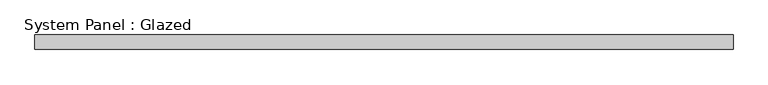
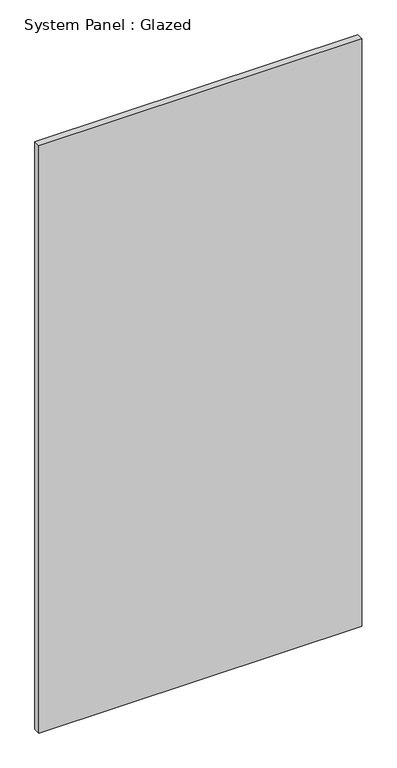
"""IFC4 building model written with IfcOpenShell, lengths in millimetres: plate geometry, System Panel : Glazed."""

from ifc_helpers import new_model, si_unit, origin, origin_with_axes, place, context, project, spatial, polyline, outline, extrude, source, transform, mapped, element, save


def system_panel_glazed_ecda40cd(model_context):
    return source(origin(), model_context, "Body", "SweptSolid", [
        extrude(outline(polyline([(609.5999999, -44.45), (-609.5999999, -44.45), (-609.5999999, -19.05), (609.5999999, -19.05), (609.5999999, -44.45)])), origin_with_axes(), (0.0, 0.0, 1.0), 2343.15),
    ])


if __name__ == "__main__":
    model = new_model("IFC4")
    model_context = context("Model", 3, world=origin())
    ifc_project = project(units=[si_unit("LENGTHUNIT", "METRE", prefix="MILLI")], contexts=[model_context])
    site = spatial("IfcSite", under=ifc_project)
    building = spatial("IfcBuilding", under=site)
    placement = place(None, origin())
    system_panel_glazed_shape = system_panel_glazed_ecda40cd(model_context)
    element("IfcPlate", 1, ObjectType="System Panel : Glazed", at=placement, inside=building, context=model_context, shape_type="MappedRepresentation", body=[
        mapped(system_panel_glazed_shape, transform((0.0, 0.0, 0.0), x_axis=(1.0, 0.0, 0.0), y_axis=(0.0, 1.0, 0.0), z_axis=(0.0, 0.0, 1.0))),
    ])
    save(model, "model.ifc")

# Revit data of these elements
# Type "System Panel : Glazed"
#   Construction Type Id = "GSP4R"
#   Analytic Construction = "1/8 in Pilkington single glazing"
#   Visual Light Transmittance = 0.9
#   Solar Heat Gain Coefficient = 0.86
#   Heat Transfer Coefficient (U) = 1.18115 BTU/(h·ft²·°F)
#   Define Thermal Properties by = 1
# Element 1 (IfcPlate, "System Panel : Glazed")
#   Materials on its faces: "glass panel 223"
# Materials
#   "glass panel 223": class "Generic", colour RGB 120 120 120, transparency 0, Cost = 0
